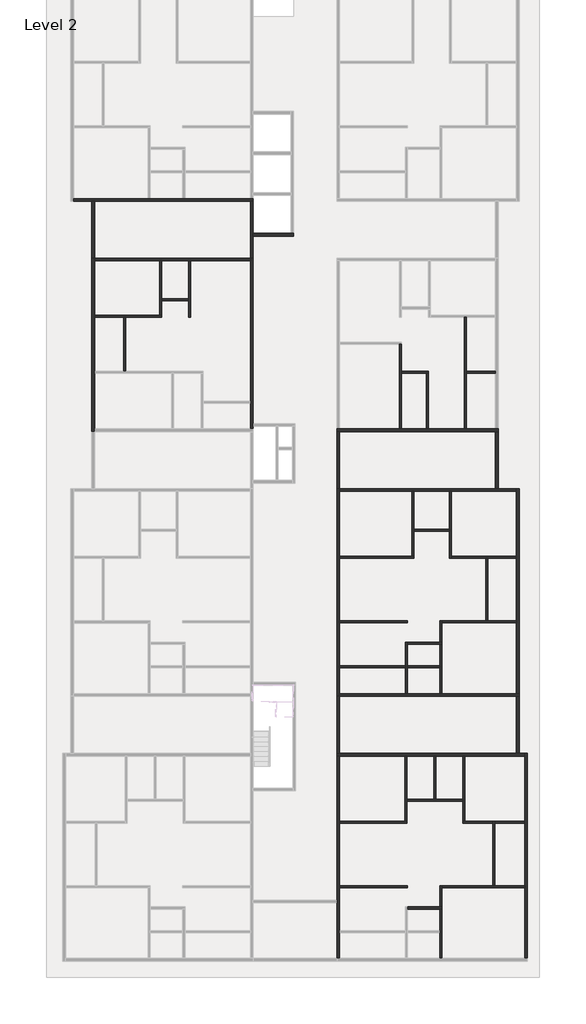
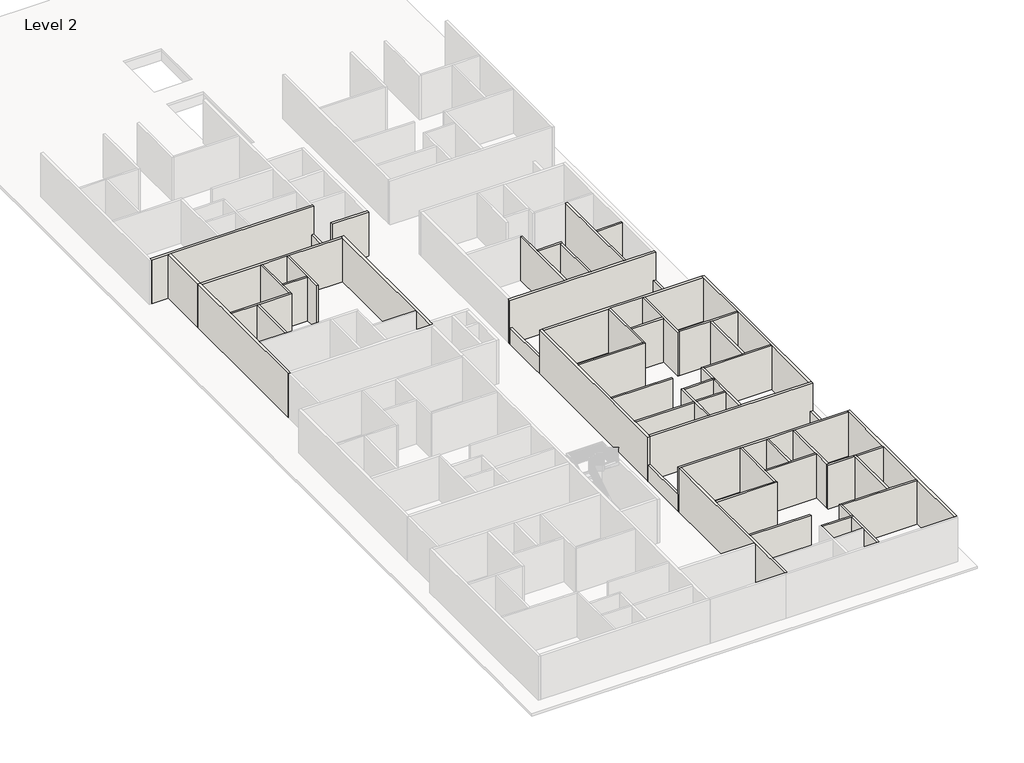
# One storey, part 2 of 8: 56 walls.
"""IFC4 building model written with IfcOpenShell, lengths in millimetres."""

from ifc_helpers import new_model, si_unit, frame, origin, place, context, project, spatial, polyline, outline, extrude, faceted_brep, element, save

model = new_model("IFC4")

# Units and contexts
model_context = context("Model", 3, world=origin())
ifc_project = project(units=[si_unit("LENGTHUNIT", "METRE", prefix="MILLI")], contexts=[model_context])

# Site, building, storey
site = spatial("IfcSite", under=ifc_project)
building = spatial("IfcBuilding", under=site)
storey = spatial("IfcBuildingStorey", under=building, Name="Level 2", Elevation=28282.6172466)

# Walls
placement = place(None, origin())
element("IfcWall", 1, ObjectType="4.5\"", at=placement, inside=storey, context=model_context, shape_type="Brep", body=[
    faceted_brep([(-12531.5544854, 2100.0216096, 28282.6172466), (-10907.2415084, 2100.0216096, 28282.6172466), (-10792.9415084, 2100.0216096, 28282.6172466), (-8759.6544854, 2100.0216096, 28282.6172466), (-8759.6544854, 2100.0216096, 31330.6172466), (-10792.9415084, 2100.0216096, 31330.6172466), (-10907.2415084, 2100.0216096, 31330.6172466), (-12531.5544854, 2100.0216096, 31330.6172466), (-12531.5544854, 2214.3216096, 28282.6172466), (-12531.5544854, 2214.3216096, 31330.6172466), (-8873.9544854, 2214.3216096, 31330.6172466), (-8759.6544854, 2214.3216096, 31330.6172466), (-8759.6544854, 2214.3216096, 28282.6172466), (-8873.9544854, 2214.3216096, 28282.6172466)], [[[0, 1, 2, 3, 4, 5, 6, 7]], [[8, 9, 10, 11, 12, 13]], [[3, 2, 1, 0, 8, 13, 12]], [[0, 7, 9, 8]], [[4, 3, 12, 11]], [[7, 6, 5, 4, 11, 10, 9]]]),
])
element("IfcWall", 2, ObjectType="4.5\"", at=placement, inside=storey, context=model_context, shape_type="Brep", body=[
    faceted_brep([(-8759.6544854, 2214.3216096, 28282.6172466), (-8759.6544854, 3014.4216096, 28282.6172466), (-8759.6544854, 3128.7216096, 28282.6172466), (-8759.6544854, 5264.2743917, 28282.6172466), (-8759.6544854, 5264.2743917, 31330.6172466), (-8759.6544854, 3128.7216096, 31330.6172466), (-8759.6544854, 3014.4216096, 31330.6172466), (-8759.6544854, 2214.3216096, 31330.6172466), (-8873.9544854, 2214.3216096, 28282.6172466), (-8873.9544854, 2214.3216096, 31330.6172466), (-8873.9544854, 5264.2743917, 31330.6172466), (-8873.9544854, 5264.2743917, 28282.6172466)], [[[0, 1, 2, 3, 4, 5, 6, 7]], [[8, 9, 10, 11]], [[3, 2, 1, 0, 8, 11]], [[0, 7, 9, 8]], [[4, 3, 11, 10]], [[7, 6, 5, 4, 10, 9]]]),
])
element("IfcWall", 3, ObjectType="4.5\"", at=placement, inside=storey, context=model_context, shape_type="Brep", body=[
    faceted_brep([(-7235.6544854, 5264.2743917, 28282.6172466), (-7235.6544854, 3128.7216096, 28282.6172466), (-7235.6544854, 3014.4216096, 28282.6172466), (-7235.6544854, 2100.0216096, 28282.6172466), (-7235.6544854, 2100.0216096, 31330.6172466), (-7235.6544854, 3014.4216096, 31330.6172466), (-7235.6544854, 3128.7216096, 31330.6172466), (-7235.6544854, 5264.2743917, 31330.6172466), (-7121.3544854, 5264.2743917, 28282.6172466), (-7121.3544854, 5264.2743917, 31330.6172466), (-7121.3544854, 2100.0216096, 31330.6172466), (-7121.3544854, 2100.0216096, 28282.6172466)], [[[0, 1, 2, 3, 4, 5, 6, 7]], [[8, 9, 10, 11]], [[3, 2, 1, 0, 8, 11]], [[4, 3, 11, 10]], [[0, 7, 9, 8]], [[7, 6, 5, 4, 10, 9]]]),
])
element("IfcWall", 4, ObjectType="4.5\"", at=placement, inside=storey, context=model_context, shape_type="SweptSolid", body=[
    extrude(outline(polyline([(-7235.6544854, 3014.4216096), (-8759.6544854, 3014.4216096), (-8759.6544854, 3128.7216096), (-7235.6544854, 3128.7216096), (-7235.6544854, 3014.4216096)])), frame((0.0, 0.0, 28282.6172466), z_axis=(0.0, 0.0, 1.0), x_axis=(1.0, 0.0, 0.0)), (0.0, 0.0, 1.0), 3048.0),
])
element("IfcWall", 5, ObjectType="4.5\"", at=placement, inside=storey, context=model_context, shape_type="SweptSolid", body=[
    extrude(outline(polyline([(-10907.2415084, -947.4344126), (-10907.2415084, 2100.0216096), (-10792.9415084, 2100.0216096), (-10792.9415084, -947.4344126), (-10907.2415084, -947.4344126)])), frame((0.0, 0.0, 28282.6172466), z_axis=(0.0, 0.0, 1.0), x_axis=(1.0, 0.0, 0.0)), (0.0, 0.0, 1.0), 3048.0),
])
element("IfcWall", 6, ObjectType="4.5\"", at=placement, inside=storey, context=model_context, shape_type="Brep", body=[
    faceted_brep([(5056.6584916, -31173.4344126, 28282.6172466), (6885.4584916, -31173.4344126, 28282.6172466), (6999.7584916, -31173.4344126, 28282.6172466), (6999.7584916, -31173.4344126, 31330.6172466), (6885.4584916, -31173.4344126, 31330.6172466), (5056.6584916, -31173.4344126, 31330.6172466), (5056.6584916, -31059.1344126, 28282.6172466), (5056.6584916, -31059.1344126, 31330.6172466), (6885.4584916, -31059.1344126, 31330.6172466), (6999.7584916, -31059.1344126, 31330.6172466), (6999.7584916, -31059.1344126, 28282.6172466), (6885.4584916, -31059.1344126, 28282.6172466)], [[[0, 1, 2, 3, 4, 5]], [[6, 7, 8, 9, 10, 11]], [[2, 1, 0, 6, 11, 10]], [[0, 5, 7, 6]], [[3, 2, 10, 9]], [[5, 4, 3, 9, 8, 7]]]),
])
element("IfcWall", 7, ObjectType="4.5\"", at=placement, inside=storey, context=model_context, shape_type="Brep", body=[
    faceted_brep([(6885.4584916, -31173.4344126, 28282.6172466), (6885.4584916, -32392.6344126, 28282.6172466), (6885.4584916, -32506.9344126, 28282.6172466), (6885.4584916, -33954.7344126, 28282.6172466), (6885.4584916, -33954.7344126, 31330.6172466), (6885.4584916, -32506.9344126, 31330.6172466), (6885.4584916, -32392.6344126, 31330.6172466), (6885.4584916, -31173.4344126, 31330.6172466), (6999.7584916, -31173.4344126, 28282.6172466), (6999.7584916, -31173.4344126, 31330.6172466), (6999.7584916, -33954.7344126, 31330.6172466), (6999.7584916, -33954.7344126, 28282.6172466)], [[[0, 1, 2, 3, 4, 5, 6, 7]], [[8, 9, 10, 11]], [[3, 2, 1, 0, 8, 11]], [[0, 7, 9, 8]], [[4, 3, 11, 10]], [[7, 6, 5, 4, 10, 9]]]),
])
element("IfcWall", 8, ObjectType="4.5\"", at=placement, inside=storey, context=model_context, shape_type="Brep", body=[
    faceted_brep([(6999.7584916, -31059.1344126, 28282.6172466), (6999.7584916, -29966.9344126, 28282.6172466), (6999.7584916, -29852.6344126, 28282.6172466), (6999.7584916, -29852.6344126, 31330.6172466), (6999.7584916, -29966.9344126, 31330.6172466), (6999.7584916, -31059.1344126, 31330.6172466), (6885.4584916, -31059.1344126, 28282.6172466), (6885.4584916, -31059.1344126, 31330.6172466), (6885.4584916, -29852.6344126, 31330.6172466), (6885.4584916, -29852.6344126, 28282.6172466)], [[[0, 1, 2, 3, 4, 5]], [[6, 7, 8, 9]], [[2, 1, 0, 6, 9]], [[0, 5, 7, 6]], [[3, 2, 9, 8]], [[5, 4, 3, 8, 7]]]),
])
element("IfcWall", 9, ObjectType="4.5\"", at=placement, inside=storey, context=model_context, shape_type="Brep", body=[
    faceted_brep([(6999.7584916, -29966.9344126, 28282.6172466), (11660.6584916, -29966.9344126, 28282.6172466), (11660.6584916, -29966.9344126, 31330.6172466), (6999.7584916, -29966.9344126, 31330.6172466), (6999.7584916, -29852.6344126, 28282.6172466), (6999.7584916, -29852.6344126, 31330.6172466), (9869.9584916, -29852.6344126, 31330.6172466), (9984.2584916, -29852.6344126, 31330.6172466), (11660.6584916, -29852.6344126, 31330.6172466), (11660.6584916, -29852.6344126, 28282.6172466), (9984.2584916, -29852.6344126, 28282.6172466), (9869.9584916, -29852.6344126, 28282.6172466)], [[[0, 1, 2, 3]], [[4, 5, 6, 7, 8, 9, 10, 11]], [[1, 0, 4, 11, 10, 9]], [[0, 3, 5, 4]], [[2, 1, 9, 8]], [[3, 2, 8, 7, 6, 5]]]),
])
element("IfcWall", 10, ObjectType="4.5\"", at=placement, inside=storey, context=model_context, shape_type="SweptSolid", body=[
    extrude(outline(polyline([(5056.6584916, -29966.9344126), (1259.3584916, -29966.9344126), (1259.3584916, -29852.6344126), (5056.6584916, -29852.6344126), (5056.6584916, -29966.9344126)])), frame((0.0, 0.0, 28282.6172466), z_axis=(0.0, 0.0, 1.0), x_axis=(1.0, 0.0, 0.0)), (0.0, 0.0, 1.0), 3048.0),
])
element("IfcWall", 11, ObjectType="4.5\"", at=placement, inside=storey, context=model_context, shape_type="Brep", body=[
    faceted_brep([(1259.3584916, -26347.4344126, 28282.6172466), (5031.2584916, -26347.4344126, 28282.6172466), (5031.2584916, -26347.4344126, 31330.6172466), (1259.3584916, -26347.4344126, 31330.6172466), (1259.3584916, -26233.1344126, 28282.6172466), (1259.3584916, -26233.1344126, 31330.6172466), (4916.9584916, -26233.1344126, 31330.6172466), (5031.2584916, -26233.1344126, 31330.6172466), (5031.2584916, -26233.1344126, 28282.6172466), (4916.9584916, -26233.1344126, 28282.6172466)], [[[0, 1, 2, 3]], [[4, 5, 6, 7, 8, 9]], [[1, 0, 4, 9, 8]], [[0, 3, 5, 4]], [[2, 1, 8, 7]], [[3, 2, 7, 6, 5]]]),
])
element("IfcWall", 12, ObjectType="4.5\"", at=placement, inside=storey, context=model_context, shape_type="Brep", body=[
    faceted_brep([(5031.2584916, -26233.1344126, 28282.6172466), (5031.2584916, -25128.2344126, 28282.6172466), (5031.2584916, -25013.9344126, 28282.6172466), (5031.2584916, -22575.5344126, 28282.6172466), (5031.2584916, -22575.5344126, 31330.6172466), (5031.2584916, -25013.9344126, 31330.6172466), (5031.2584916, -25128.2344126, 31330.6172466), (5031.2584916, -26233.1344126, 31330.6172466), (4916.9584916, -26233.1344126, 28282.6172466), (4916.9584916, -26233.1344126, 31330.6172466), (4916.9584916, -22575.5344126, 31330.6172466), (4916.9584916, -22575.5344126, 28282.6172466)], [[[0, 1, 2, 3, 4, 5, 6, 7]], [[8, 9, 10, 11]], [[3, 2, 1, 0, 8, 11]], [[0, 7, 9, 8]], [[4, 3, 11, 10]], [[7, 6, 5, 4, 10, 9]]]),
])
element("IfcWall", 13, ObjectType="4.5\"", at=placement, inside=storey, context=model_context, shape_type="Brep", body=[
    faceted_brep([(9984.2584916, -29852.6344126, 28282.6172466), (9984.2584916, -26347.4344126, 28282.6172466), (9984.2584916, -26233.1344126, 28282.6172466), (9984.2584916, -26233.1344126, 31330.6172466), (9984.2584916, -26347.4344126, 31330.6172466), (9984.2584916, -29852.6344126, 31330.6172466), (9869.9584916, -29852.6344126, 28282.6172466), (9869.9584916, -29852.6344126, 31330.6172466), (9869.9584916, -26347.4344126, 31330.6172466), (9869.9584916, -26233.1344126, 31330.6172466), (9869.9584916, -26233.1344126, 28282.6172466), (9869.9584916, -26347.4344126, 28282.6172466)], [[[0, 1, 2, 3, 4, 5]], [[6, 7, 8, 9, 10, 11]], [[2, 1, 0, 6, 11, 10]], [[0, 5, 7, 6]], [[3, 2, 10, 9]], [[5, 4, 3, 9, 8, 7]]]),
])
element("IfcWall", 14, ObjectType="4.5\"", at=placement, inside=storey, context=model_context, shape_type="SweptSolid", body=[
    extrude(outline(polyline([(11660.6584916, -26347.4344126), (9984.2584916, -26347.4344126), (9984.2584916, -26233.1344126), (11660.6584916, -26233.1344126), (11660.6584916, -26347.4344126)])), frame((0.0, 0.0, 28282.6172466), z_axis=(0.0, 0.0, 1.0), x_axis=(1.0, 0.0, 0.0)), (0.0, 0.0, 1.0), 3048.0),
])
element("IfcWall", 15, ObjectType="4.5\"", at=placement, inside=storey, context=model_context, shape_type="Brep", body=[
    faceted_brep([(9869.9584916, -26233.1344126, 28282.6172466), (8307.8584916, -26233.1344126, 28282.6172466), (8193.5584916, -26233.1344126, 28282.6172466), (8193.5584916, -26233.1344126, 31330.6172466), (8307.8584916, -26233.1344126, 31330.6172466), (9869.9584916, -26233.1344126, 31330.6172466), (9869.9584916, -26347.4344126, 28282.6172466), (9869.9584916, -26347.4344126, 31330.6172466), (8193.5584916, -26347.4344126, 31330.6172466), (8193.5584916, -26347.4344126, 28282.6172466)], [[[0, 1, 2, 3, 4, 5]], [[6, 7, 8, 9]], [[2, 1, 0, 6, 9]], [[0, 5, 7, 6]], [[3, 2, 9, 8]], [[5, 4, 3, 8, 7]]]),
])
element("IfcWall", 16, ObjectType="4.5\"", at=placement, inside=storey, context=model_context, shape_type="Brep", body=[
    faceted_brep([(8307.8584916, -26233.1344126, 28282.6172466), (8307.8584916, -22575.5344126, 28282.6172466), (8307.8584916, -22575.5344126, 31330.6172466), (8307.8584916, -26233.1344126, 31330.6172466), (8193.5584916, -26233.1344126, 28282.6172466), (8193.5584916, -26233.1344126, 31330.6172466), (8193.5584916, -25128.2344126, 31330.6172466), (8193.5584916, -25013.9344126, 31330.6172466), (8193.5584916, -22575.5344126, 31330.6172466), (8193.5584916, -22575.5344126, 28282.6172466), (8193.5584916, -25013.9344126, 28282.6172466), (8193.5584916, -25128.2344126, 28282.6172466)], [[[0, 1, 2, 3]], [[4, 5, 6, 7, 8, 9, 10, 11]], [[1, 0, 4, 11, 10, 9]], [[0, 3, 5, 4]], [[2, 1, 9, 8]], [[3, 2, 8, 7, 6, 5]]]),
])
element("IfcWall", 17, ObjectType="4.5\"", at=placement, inside=storey, context=model_context, shape_type="Brep", body=[
    faceted_brep([(5031.2584916, -25128.2344126, 28282.6172466), (8193.5584916, -25128.2344126, 28282.6172466), (8193.5584916, -25128.2344126, 31330.6172466), (5031.2584916, -25128.2344126, 31330.6172466), (5031.2584916, -25013.9344126, 28282.6172466), (5031.2584916, -25013.9344126, 31330.6172466), (6555.2584916, -25013.9344126, 31330.6172466), (6669.5584916, -25013.9344126, 31330.6172466), (8193.5584916, -25013.9344126, 31330.6172466), (8193.5584916, -25013.9344126, 28282.6172466), (6669.5584916, -25013.9344126, 28282.6172466), (6555.2584916, -25013.9344126, 28282.6172466)], [[[0, 1, 2, 3]], [[4, 5, 6, 7, 8, 9, 10, 11]], [[1, 0, 4, 11, 10, 9]], [[0, 3, 5, 4]], [[2, 1, 9, 8]], [[3, 2, 8, 7, 6, 5]]]),
])
element("IfcWall", 18, ObjectType="4.5\"", at=placement, inside=storey, context=model_context, shape_type="SweptSolid", body=[
    extrude(outline(polyline([(6555.2584916, -25013.9344126), (6555.2584916, -22575.5344126), (6669.5584916, -22575.5344126), (6669.5584916, -25013.9344126), (6555.2584916, -25013.9344126)])), frame((0.0, 0.0, 28282.6172466), z_axis=(0.0, 0.0, 1.0), x_axis=(1.0, 0.0, 0.0)), (0.0, 0.0, 1.0), 3048.0),
])
element("IfcWall", 19, ObjectType="4.5\"", at=placement, inside=storey, context=model_context, shape_type="SweptSolid", body=[
    extrude(outline(polyline([(4942.3584916, -17622.5344126), (1259.3584916, -17622.5344126), (1259.3584916, -17508.2344126), (4942.3584916, -17508.2344126), (4942.3584916, -17622.5344126)])), frame((0.0, 0.0, 28282.6172466), z_axis=(0.0, 0.0, 1.0), x_axis=(1.0, 0.0, 0.0)), (0.0, 0.0, 1.0), 3048.0),
])
element("IfcWall", 20, ObjectType="4.5\"", at=placement, inside=storey, context=model_context, shape_type="Brep", body=[
    faceted_brep([(4942.3584916, -16174.7344126, 28282.6172466), (4942.3584916, -17508.2344126, 28282.6172466), (4942.3584916, -17622.5344126, 28282.6172466), (4942.3584916, -19070.3344126, 28282.6172466), (4942.3584916, -19070.3344126, 31330.6172466), (4942.3584916, -17622.5344126, 31330.6172466), (4942.3584916, -17508.2344126, 31330.6172466), (4942.3584916, -16174.7344126, 31330.6172466), (5056.6584916, -16174.7344126, 28282.6172466), (5056.6584916, -16174.7344126, 31330.6172466), (5056.6584916, -16289.0344126, 31330.6172466), (5056.6584916, -17508.2344126, 31330.6172466), (5056.6584916, -17622.5344126, 31330.6172466), (5056.6584916, -19070.3344126, 31330.6172466), (5056.6584916, -19070.3344126, 28282.6172466), (5056.6584916, -17622.5344126, 28282.6172466), (5056.6584916, -17508.2344126, 28282.6172466), (5056.6584916, -16289.0344126, 28282.6172466)], [[[0, 1, 2, 3, 4, 5, 6, 7]], [[8, 9, 10, 11, 12, 13, 14, 15, 16, 17]], [[3, 2, 1, 0, 8, 17, 16, 15, 14]], [[4, 3, 14, 13]], [[0, 7, 9, 8]], [[7, 6, 5, 4, 13, 12, 11, 10, 9]]]),
])
element("IfcWall", 21, ObjectType="4.5\"", at=placement, inside=storey, context=model_context, shape_type="Brep", body=[
    faceted_brep([(5056.6584916, -16289.0344126, 28282.6172466), (6885.4584916, -16289.0344126, 28282.6172466), (6999.7584916, -16289.0344126, 28282.6172466), (6999.7584916, -16289.0344126, 31330.6172466), (6885.4584916, -16289.0344126, 31330.6172466), (5056.6584916, -16289.0344126, 31330.6172466), (5056.6584916, -16174.7344126, 28282.6172466), (5056.6584916, -16174.7344126, 31330.6172466), (6885.4584916, -16174.7344126, 31330.6172466), (6999.7584916, -16174.7344126, 31330.6172466), (6999.7584916, -16174.7344126, 28282.6172466), (6885.4584916, -16174.7344126, 28282.6172466)], [[[0, 1, 2, 3, 4, 5]], [[6, 7, 8, 9, 10, 11]], [[2, 1, 0, 6, 11, 10]], [[0, 5, 7, 6]], [[3, 2, 10, 9]], [[5, 4, 3, 9, 8, 7]]]),
])
element("IfcWall", 22, ObjectType="4.5\"", at=placement, inside=storey, context=model_context, shape_type="Brep", body=[
    faceted_brep([(6885.4584916, -16289.0344126, 28282.6172466), (6885.4584916, -17508.2344126, 28282.6172466), (6885.4584916, -17622.5344126, 28282.6172466), (6885.4584916, -19070.3344126, 28282.6172466), (6885.4584916, -19070.3344126, 31330.6172466), (6885.4584916, -17622.5344126, 31330.6172466), (6885.4584916, -17508.2344126, 31330.6172466), (6885.4584916, -16289.0344126, 31330.6172466), (6999.7584916, -16289.0344126, 28282.6172466), (6999.7584916, -16289.0344126, 31330.6172466), (6999.7584916, -19070.3344126, 31330.6172466), (6999.7584916, -19070.3344126, 28282.6172466)], [[[0, 1, 2, 3, 4, 5, 6, 7]], [[8, 9, 10, 11]], [[3, 2, 1, 0, 8, 11]], [[0, 7, 9, 8]], [[4, 3, 11, 10]], [[7, 6, 5, 4, 10, 9]]]),
])
element("IfcWall", 23, ObjectType="4.5\"", at=placement, inside=storey, context=model_context, shape_type="SweptSolid", body=[
    extrude(outline(polyline([(6885.4584916, -17622.5344126), (5056.6584916, -17622.5344126), (5056.6584916, -17508.2344126), (6885.4584916, -17508.2344126), (6885.4584916, -17622.5344126)])), frame((0.0, 0.0, 28282.6172466), z_axis=(0.0, 0.0, 1.0), x_axis=(1.0, 0.0, 0.0)), (0.0, 0.0, 1.0), 3048.0),
])
element("IfcWall", 24, ObjectType="4.5\"", at=placement, inside=storey, context=model_context, shape_type="Brep", body=[
    faceted_brep([(6999.7584916, -16174.7344126, 28282.6172466), (6999.7584916, -15082.5344126, 28282.6172466), (6999.7584916, -14968.2344126, 28282.6172466), (6999.7584916, -14968.2344126, 31330.6172466), (6999.7584916, -15082.5344126, 31330.6172466), (6999.7584916, -16174.7344126, 31330.6172466), (6885.4584916, -16174.7344126, 28282.6172466), (6885.4584916, -16174.7344126, 31330.6172466), (6885.4584916, -14968.2344126, 31330.6172466), (6885.4584916, -14968.2344126, 28282.6172466)], [[[0, 1, 2, 3, 4, 5]], [[6, 7, 8, 9]], [[2, 1, 0, 6, 9]], [[0, 5, 7, 6]], [[3, 2, 9, 8]], [[5, 4, 3, 8, 7]]]),
])
element("IfcWall", 25, ObjectType="4.5\"", at=placement, inside=storey, context=model_context, shape_type="Brep", body=[
    faceted_brep([(6999.7584916, -15082.5344126, 28282.6172466), (11208.5214687, -15082.5344126, 28282.6172466), (11208.5214687, -15082.5344126, 31330.6172466), (6999.7584916, -15082.5344126, 31330.6172466), (6999.7584916, -14968.2344126, 28282.6172466), (6999.7584916, -14968.2344126, 31330.6172466), (9469.9084916, -14968.2344126, 31330.6172466), (9584.2084916, -14968.2344126, 31330.6172466), (11208.5214687, -14968.2344126, 31330.6172466), (11208.5214687, -14968.2344126, 28282.6172466), (9584.2084916, -14968.2344126, 28282.6172466), (9469.9084916, -14968.2344126, 28282.6172466)], [[[0, 1, 2, 3]], [[4, 5, 6, 7, 8, 9, 10, 11]], [[1, 0, 4, 11, 10, 9]], [[0, 3, 5, 4]], [[2, 1, 9, 8]], [[3, 2, 8, 7, 6, 5]]]),
])
element("IfcWall", 26, ObjectType="4.5\"", at=placement, inside=storey, context=model_context, shape_type="SweptSolid", body=[
    extrude(outline(polyline([(5056.6584916, -15082.5344126), (1259.3584916, -15082.5344126), (1259.3584916, -14968.2344126), (5056.6584916, -14968.2344126), (5056.6584916, -15082.5344126)])), frame((0.0, 0.0, 28282.6172466), z_axis=(0.0, 0.0, 1.0), x_axis=(1.0, 0.0, 0.0)), (0.0, 0.0, 1.0), 3048.0),
])
element("IfcWall", 27, ObjectType="4.5\"", at=placement, inside=storey, context=model_context, shape_type="Brep", body=[
    faceted_brep([(1259.3584916, -11463.0344126, 28282.6172466), (5430.0214687, -11463.0344126, 28282.6172466), (5430.0214687, -11463.0344126, 31330.6172466), (1259.3584916, -11463.0344126, 31330.6172466), (1259.3584916, -11348.7344126, 28282.6172466), (1259.3584916, -11348.7344126, 31330.6172466), (5315.7214687, -11348.7344126, 31330.6172466), (5430.0214687, -11348.7344126, 31330.6172466), (5430.0214687, -11348.7344126, 28282.6172466), (5315.7214687, -11348.7344126, 28282.6172466)], [[[0, 1, 2, 3]], [[4, 5, 6, 7, 8, 9]], [[1, 0, 4, 9, 8]], [[0, 3, 5, 4]], [[2, 1, 8, 7]], [[3, 2, 7, 6, 5]]]),
])
element("IfcWall", 28, ObjectType="4.5\"", at=placement, inside=storey, context=model_context, shape_type="Brep", body=[
    faceted_brep([(5430.0214687, -11348.7344126, 28282.6172466), (5430.0214687, -9939.0344126, 28282.6172466), (5430.0214687, -9824.7344126, 28282.6172466), (5430.0214687, -7691.1344126, 28282.6172466), (5430.0214687, -7691.1344126, 31330.6172466), (5430.0214687, -9824.7344126, 31330.6172466), (5430.0214687, -9939.0344126, 31330.6172466), (5430.0214687, -11348.7344126, 31330.6172466), (5315.7214687, -11348.7344126, 28282.6172466), (5315.7214687, -11348.7344126, 31330.6172466), (5315.7214687, -7691.1344126, 31330.6172466), (5315.7214687, -7691.1344126, 28282.6172466)], [[[0, 1, 2, 3, 4, 5, 6, 7]], [[8, 9, 10, 11]], [[3, 2, 1, 0, 8, 11]], [[0, 7, 9, 8]], [[4, 3, 11, 10]], [[7, 6, 5, 4, 10, 9]]]),
])
element("IfcWall", 29, ObjectType="4.5\"", at=placement, inside=storey, context=model_context, shape_type="SweptSolid", body=[
    extrude(outline(polyline([(7436.6214687, -9939.0344126), (5430.0214687, -9939.0344126), (5430.0214687, -9824.7344126), (7436.6214687, -9824.7344126), (7436.6214687, -9939.0344126)])), frame((0.0, 0.0, 28282.6172466), z_axis=(0.0, 0.0, 1.0), x_axis=(1.0, 0.0, 0.0)), (0.0, 0.0, 1.0), 3048.0),
])
element("IfcWall", 30, ObjectType="4.5\"", at=placement, inside=storey, context=model_context, shape_type="Brep", body=[
    faceted_brep([(7436.6214687, -7691.1344126, 28282.6172466), (7436.6214687, -9824.7344126, 28282.6172466), (7436.6214687, -9939.0344126, 28282.6172466), (7436.6214687, -11463.0344126, 28282.6172466), (7436.6214687, -11463.0344126, 31330.6172466), (7436.6214687, -9939.0344126, 31330.6172466), (7436.6214687, -9824.7344126, 31330.6172466), (7436.6214687, -7691.1344126, 31330.6172466), (7550.9214687, -7691.1344126, 28282.6172466), (7550.9214687, -7691.1344126, 31330.6172466), (7550.9214687, -11348.7344126, 31330.6172466), (7550.9214687, -11463.0344126, 31330.6172466), (7550.9214687, -11463.0344126, 28282.6172466), (7550.9214687, -11348.7344126, 28282.6172466)], [[[0, 1, 2, 3, 4, 5, 6, 7]], [[8, 9, 10, 11, 12, 13]], [[3, 2, 1, 0, 8, 13, 12]], [[0, 7, 9, 8]], [[4, 3, 12, 11]], [[7, 6, 5, 4, 11, 10, 9]]]),
])
element("IfcWall", 31, ObjectType="4.5\"", at=placement, inside=storey, context=model_context, shape_type="Brep", body=[
    faceted_brep([(7550.9214687, -11463.0344126, 28282.6172466), (9469.9084916, -11463.0344126, 28282.6172466), (9584.2084916, -11463.0344126, 28282.6172466), (11208.5214687, -11463.0344126, 28282.6172466), (11208.5214687, -11463.0344126, 31330.6172466), (9584.2084916, -11463.0344126, 31330.6172466), (9469.9084916, -11463.0344126, 31330.6172466), (7550.9214687, -11463.0344126, 31330.6172466), (7550.9214687, -11348.7344126, 28282.6172466), (7550.9214687, -11348.7344126, 31330.6172466), (11208.5214687, -11348.7344126, 31330.6172466), (11208.5214687, -11348.7344126, 28282.6172466)], [[[0, 1, 2, 3, 4, 5, 6, 7]], [[8, 9, 10, 11]], [[3, 2, 1, 0, 8, 11]], [[0, 7, 9, 8]], [[4, 3, 11, 10]], [[7, 6, 5, 4, 10, 9]]]),
])
element("IfcWall", 32, ObjectType="4.5\"", at=placement, inside=storey, context=model_context, shape_type="SweptSolid", body=[
    extrude(outline(polyline([(9469.9084916, -14968.2344126), (9469.9084916, -11463.0344126), (9584.2084916, -11463.0344126), (9584.2084916, -14968.2344126), (9469.9084916, -14968.2344126)])), frame((0.0, 0.0, 28282.6172466), z_axis=(0.0, 0.0, 1.0), x_axis=(1.0, 0.0, 0.0)), (0.0, 0.0, 1.0), 3048.0),
])
element("IfcWall", 33, ObjectType="4.5\"", at=placement, inside=storey, context=model_context, shape_type="Brep", body=[
    faceted_brep([(4610.8714687, 572.7745083, 28282.6172466), (4610.8714687, -4185.9344126, 28282.6172466), (4610.8714687, -4185.9344126, 31330.6172466), (4610.8714687, 572.7745083, 31330.6172466), (4725.1714687, 572.7745083, 28282.6172466), (4725.1714687, 572.7745083, 31330.6172466), (4725.1714687, -947.4344126, 31330.6172466), (4725.1714687, -1061.7344126, 31330.6172466), (4725.1714687, -4185.9344126, 31330.6172466), (4725.1714687, -4185.9344126, 28282.6172466), (4725.1714687, -1061.7344126, 28282.6172466), (4725.1714687, -947.4344126, 28282.6172466)], [[[0, 1, 2, 3]], [[4, 5, 6, 7, 8, 9, 10, 11]], [[1, 0, 4, 11, 10, 9]], [[0, 3, 5, 4]], [[2, 1, 9, 8]], [[3, 2, 8, 7, 6, 5]]]),
])
element("IfcWall", 34, ObjectType="4.5\"", at=placement, inside=storey, context=model_context, shape_type="Brep", body=[
    faceted_brep([(4725.1714687, -1061.7344126, 28282.6172466), (6134.8714687, -1061.7344126, 28282.6172466), (6249.1714687, -1061.7344126, 28282.6172466), (6249.1714687, -1061.7344126, 31330.6172466), (6134.8714687, -1061.7344126, 31330.6172466), (4725.1714687, -1061.7344126, 31330.6172466), (4725.1714687, -947.4344126, 28282.6172466), (4725.1714687, -947.4344126, 31330.6172466), (6249.1714687, -947.4344126, 31330.6172466), (6249.1714687, -947.4344126, 28282.6172466)], [[[0, 1, 2, 3, 4, 5]], [[6, 7, 8, 9]], [[2, 1, 0, 6, 9]], [[0, 5, 7, 6]], [[3, 2, 9, 8]], [[5, 4, 3, 8, 7]]]),
])
element("IfcWall", 35, ObjectType="4.5\"", at=placement, inside=storey, context=model_context, shape_type="SweptSolid", body=[
    extrude(outline(polyline([(6134.8714687, -4185.9344126), (6134.8714687, -1061.7344126), (6249.1714687, -1061.7344126), (6249.1714687, -4185.9344126), (6134.8714687, -4185.9344126)])), frame((0.0, 0.0, 28282.6172466), z_axis=(0.0, 0.0, 1.0), x_axis=(1.0, 0.0, 0.0)), (0.0, 0.0, 1.0), 3048.0),
])
element("IfcWall", 36, ObjectType="4.5\"", at=placement, inside=storey, context=model_context, shape_type="Brep", body=[
    faceted_brep([(8396.7584916, -4185.9344126, 28282.6172466), (8396.7584916, -1061.7344126, 28282.6172466), (8396.7584916, -947.4344126, 28282.6172466), (8396.7584916, 2100.0216096, 28282.6172466), (8396.7584916, 2100.0216096, 31330.6172466), (8396.7584916, -947.4344126, 31330.6172466), (8396.7584916, -1061.7344126, 31330.6172466), (8396.7584916, -4185.9344126, 31330.6172466), (8282.4584916, -4185.9344126, 28282.6172466), (8282.4584916, -4185.9344126, 31330.6172466), (8282.4584916, 2100.0216096, 31330.6172466), (8282.4584916, 2100.0216096, 28282.6172466)], [[[0, 1, 2, 3, 4, 5, 6, 7]], [[8, 9, 10, 11]], [[3, 2, 1, 0, 8, 11]], [[0, 7, 9, 8]], [[4, 3, 11, 10]], [[7, 6, 5, 4, 10, 9]]]),
])
element("IfcWall", 37, ObjectType="4.5\"", at=placement, inside=storey, context=model_context, shape_type="SweptSolid", body=[
    extrude(outline(polyline([(8396.7584916, -947.4344126), (10021.0714687, -947.4344126), (10021.0714687, -1061.7344126), (8396.7584916, -1061.7344126), (8396.7584916, -947.4344126)])), frame((0.0, 0.0, 28282.6172466), z_axis=(0.0, 0.0, 1.0), x_axis=(1.0, 0.0, 0.0)), (0.0, 0.0, 1.0), 3048.0),
])
element("IfcWall", 38, ObjectType="6\"", at=placement, inside=storey, context=model_context, shape_type="Brep", body=[
    faceted_brep([(-13719.0044854, 8615.1216096, 28282.6172466), (-12683.9544854, 8615.1216096, 28282.6172466), (-12531.5544854, 8615.1216096, 28282.6172466), (-3769.8415084, 8615.1216096, 28282.6172466), (-3617.4415084, 8615.1216096, 28282.6172466), (-3617.4415084, 8615.1216096, 29501.8172466), (-3617.4415084, 8615.1216096, 31330.6172466), (-12531.5544854, 8615.1216096, 31330.6172466), (-12683.9544854, 8615.1216096, 31330.6172466), (-13719.0044854, 8615.1216096, 31330.6172466), (-13719.0044854, 8767.5216096, 28282.6172466), (-13719.0044854, 8767.5216096, 31330.6172466), (-9510.2415084, 8767.5216096, 31330.6172466), (-9395.9415084, 8767.5216096, 31330.6172466), (-7567.1415084, 8767.5216096, 31330.6172466), (-7452.8415084, 8767.5216096, 31330.6172466), (-3769.8415084, 8767.5216096, 31330.6172466), (-3617.4415084, 8767.5216096, 31330.6172466), (-3617.4415084, 8767.5216096, 28282.6172466), (-3769.8415084, 8767.5216096, 28282.6172466), (-7452.8415084, 8767.5216096, 28282.6172466), (-7567.1415084, 8767.5216096, 28282.6172466), (-9395.9415084, 8767.5216096, 28282.6172466), (-9510.2415084, 8767.5216096, 28282.6172466)], [[[0, 1, 2, 3, 4, 5, 6, 7, 8, 9]], [[10, 11, 12, 13, 14, 15, 16, 17, 18, 19, 20, 21, 22, 23]], [[4, 3, 2, 1, 0, 10, 23, 22, 21, 20, 19, 18]], [[0, 9, 11, 10]], [[4, 18, 17, 6, 5]], [[9, 8, 7, 6, 17, 16, 15, 14, 13, 12, 11]]]),
])
element("IfcWall", 39, ObjectType="6\"", at=placement, inside=storey, context=model_context, shape_type="Brep", body=[
    faceted_brep([(-12683.9544854, 5416.6743917, 28282.6172466), (-12683.9544854, -4338.3344126, 28282.6172466), (-12683.9544854, -4338.3344126, 31330.6172466), (-12683.9544854, 5416.6743917, 31330.6172466), (-12531.5544854, 5416.6743917, 28282.6172466), (-12531.5544854, 5416.6743917, 31330.6172466), (-12531.5544854, 5264.2743917, 31330.6172466), (-12531.5544854, 2214.3216096, 31330.6172466), (-12531.5544854, 2100.0216096, 31330.6172466), (-12531.5544854, -947.4344126, 31330.6172466), (-12531.5544854, -1061.7344126, 31330.6172466), (-12531.5544854, -4185.9344126, 31330.6172466), (-12531.5544854, -4338.3344126, 31330.6172466), (-12531.5544854, -4338.3344126, 28282.6172466), (-12531.5544854, -4185.9344126, 28282.6172466), (-12531.5544854, -1061.7344126, 28282.6172466), (-12531.5544854, -947.4344126, 28282.6172466), (-12531.5544854, 2100.0216096, 28282.6172466), (-12531.5544854, 2214.3216096, 28282.6172466), (-12531.5544854, 5264.2743917, 28282.6172466)], [[[0, 1, 2, 3]], [[4, 5, 6, 7, 8, 9, 10, 11, 12, 13, 14, 15, 16, 17, 18, 19]], [[1, 0, 4, 19, 18, 17, 16, 15, 14, 13]], [[2, 1, 13, 12]], [[0, 3, 5, 4]], [[3, 2, 12, 11, 10, 9, 8, 7, 6, 5]]]),
])
element("IfcWall", 40, ObjectType="6\"", at=placement, inside=storey, context=model_context, shape_type="Brep", body=[
    faceted_brep([(-3617.4415084, -4185.9344126, 28282.6172466), (-3617.4415084, -4034.6751812, 28282.6172466), (-3617.4415084, -3882.2751812, 28282.6172466), (-3617.4415084, 5416.6743917, 28282.6172466), (-3617.4415084, 5416.6743917, 31330.6172466), (-3617.4415084, -3882.2751812, 31330.6172466), (-3617.4415084, -4034.6751812, 31330.6172466), (-3617.4415084, -4185.9344126, 31330.6172466), (-3769.8415084, -4185.9344126, 28282.6172466), (-3769.8415084, -4185.9344126, 31330.6172466), (-3769.8415084, -2738.1344126, 31330.6172466), (-3769.8415084, -2623.8344126, 31330.6172466), (-3769.8415084, 5264.2743917, 31330.6172466), (-3769.8415084, 5416.6743917, 31330.6172466), (-3769.8415084, 5416.6743917, 28282.6172466), (-3769.8415084, 5264.2743917, 28282.6172466), (-3769.8415084, -2623.8344126, 28282.6172466), (-3769.8415084, -2738.1344126, 28282.6172466)], [[[0, 1, 2, 3, 4, 5, 6, 7]], [[8, 9, 10, 11, 12, 13, 14, 15, 16, 17]], [[3, 2, 1, 0, 8, 17, 16, 15, 14]], [[0, 7, 9, 8]], [[3, 14, 13, 4]], [[7, 6, 5, 4, 13, 12, 11, 10, 9]]]),
])
element("IfcWall", 41, ObjectType="6\"", at=placement, inside=storey, context=model_context, shape_type="Brep", body=[
    faceted_brep([(-3769.8415084, 5416.6743917, 31330.6172466), (-3769.8415084, 5416.6743917, 28282.6172466), (-12531.5544854, 5416.6743917, 28282.6172466), (-12531.5544854, 5416.6743917, 31330.6172466), (-3769.8415084, 5264.2743917, 28282.6172466), (-3769.8415084, 5264.2743917, 31330.6172466), (-7121.3544854, 5264.2743917, 31330.6172466), (-7235.6544854, 5264.2743917, 31330.6172466), (-8759.6544854, 5264.2743917, 31330.6172466), (-8873.9544854, 5264.2743917, 31330.6172466), (-12531.5544854, 5264.2743917, 31330.6172466), (-12531.5544854, 5264.2743917, 28282.6172466), (-8873.9544854, 5264.2743917, 28282.6172466), (-8759.6544854, 5264.2743917, 28282.6172466), (-7235.6544854, 5264.2743917, 28282.6172466), (-7121.3544854, 5264.2743917, 28282.6172466)], [[[0, 1, 2, 3]], [[4, 5, 6, 7, 8, 9, 10, 11, 12, 13, 14, 15]], [[2, 1, 4, 15, 14, 13, 12, 11]], [[3, 2, 11, 10]], [[0, 5, 4, 1]], [[0, 3, 10, 9, 8, 7, 6, 5]]]),
])
element("IfcWall", 42, ObjectType="6\"", at=placement, inside=storey, context=model_context, shape_type="Brep", body=[
    faceted_brep([(11813.0584916, -33954.7344126, 28282.6172466), (11813.0584916, -22423.1344126, 28282.6172466), (11813.0584916, -22423.1344126, 31330.6172466), (11813.0584916, -33954.7344126, 31330.6172466), (11660.6584916, -33954.7344126, 28282.6172466), (11660.6584916, -33954.7344126, 31330.6172466), (11660.6584916, -29966.9344126, 31330.6172466), (11660.6584916, -29852.6344126, 31330.6172466), (11660.6584916, -26347.4344126, 31330.6172466), (11660.6584916, -26233.1344126, 31330.6172466), (11660.6584916, -22575.5344126, 31330.6172466), (11660.6584916, -22423.1344126, 31330.6172466), (11660.6584916, -22423.1344126, 28282.6172466), (11660.6584916, -22575.5344126, 28282.6172466), (11660.6584916, -26233.1344126, 28282.6172466), (11660.6584916, -26347.4344126, 28282.6172466), (11660.6584916, -29852.6344126, 28282.6172466), (11660.6584916, -29966.9344126, 28282.6172466)], [[[0, 1, 2, 3]], [[4, 5, 6, 7, 8, 9, 10, 11, 12, 13, 14, 15, 16, 17]], [[1, 0, 4, 17, 16, 15, 14, 13, 12]], [[0, 3, 5, 4]], [[2, 1, 12, 11]], [[3, 2, 11, 10, 9, 8, 7, 6, 5]]]),
])
element("IfcWall", 43, ObjectType="6\"", at=placement, inside=storey, context=model_context, shape_type="Brep", body=[
    faceted_brep([(11660.6584916, -22423.1344126, 28282.6172466), (11360.9214687, -22423.1344126, 28282.6172466), (11208.5214687, -22423.1344126, 28282.6172466), (1259.3584916, -22423.1344126, 28282.6172466), (1106.9584916, -22423.1344126, 28282.6172466), (1106.9584916, -22423.1344126, 29501.8172466), (1106.9584916, -22423.1344126, 31330.6172466), (11660.6584916, -22423.1344126, 31330.6172466), (11660.6584916, -22575.5344126, 28282.6172466), (11660.6584916, -22575.5344126, 31330.6172466), (8307.8584916, -22575.5344126, 31330.6172466), (8193.5584916, -22575.5344126, 31330.6172466), (6669.5584916, -22575.5344126, 31330.6172466), (6555.2584916, -22575.5344126, 31330.6172466), (5031.2584916, -22575.5344126, 31330.6172466), (4916.9584916, -22575.5344126, 31330.6172466), (1259.3584916, -22575.5344126, 31330.6172466), (1106.9584916, -22575.5344126, 31330.6172466), (1106.9584916, -22575.5344126, 28282.6172466), (1259.3584916, -22575.5344126, 28282.6172466), (4916.9584916, -22575.5344126, 28282.6172466), (5031.2584916, -22575.5344126, 28282.6172466), (6555.2584916, -22575.5344126, 28282.6172466), (6669.5584916, -22575.5344126, 28282.6172466), (8193.5584916, -22575.5344126, 28282.6172466), (8307.8584916, -22575.5344126, 28282.6172466)], [[[0, 1, 2, 3, 4, 5, 6, 7]], [[8, 9, 10, 11, 12, 13, 14, 15, 16, 17, 18, 19, 20, 21, 22, 23, 24, 25]], [[4, 3, 2, 1, 0, 8, 25, 24, 23, 22, 21, 20, 19, 18]], [[0, 7, 9, 8]], [[4, 18, 17, 6, 5]], [[7, 6, 17, 16, 15, 14, 13, 12, 11, 10, 9]]]),
])
element("IfcWall", 44, ObjectType="6\"", at=placement, inside=storey, context=model_context, shape_type="Brep", body=[
    faceted_brep([(1106.9584916, -22575.5344126, 31330.6172466), (1106.9584916, -22575.5344126, 28282.6172466), (1106.9584916, -30668.5325185, 28282.6172466), (1106.9584916, -30820.9325185, 28282.6172466), (1106.9584916, -33954.7344126, 28282.6172466), (1106.9584916, -33954.7344126, 31330.6172466), (1106.9584916, -30820.9325185, 31330.6172466), (1106.9584916, -30668.5325185, 31330.6172466), (1259.3584916, -22575.5344126, 28282.6172466), (1259.3584916, -22575.5344126, 31330.6172466), (1259.3584916, -26233.1344126, 31330.6172466), (1259.3584916, -26347.4344126, 31330.6172466), (1259.3584916, -29852.6344126, 31330.6172466), (1259.3584916, -29966.9344126, 31330.6172466), (1259.3584916, -32392.6344126, 31330.6172466), (1259.3584916, -32506.9344126, 31330.6172466), (1259.3584916, -33954.7344126, 31330.6172466), (1259.3584916, -33954.7344126, 28282.6172466), (1259.3584916, -32506.9344126, 28282.6172466), (1259.3584916, -32392.6344126, 28282.6172466), (1259.3584916, -29966.9344126, 28282.6172466), (1259.3584916, -29852.6344126, 28282.6172466), (1259.3584916, -26347.4344126, 28282.6172466), (1259.3584916, -26233.1344126, 28282.6172466)], [[[0, 1, 2, 3, 4, 5, 6, 7]], [[8, 9, 10, 11, 12, 13, 14, 15, 16, 17, 18, 19, 20, 21, 22, 23]], [[4, 3, 2, 1, 8, 23, 22, 21, 20, 19, 18, 17]], [[5, 4, 17, 16]], [[0, 9, 8, 1]], [[0, 7, 6, 5, 16, 15, 14, 13, 12, 11, 10, 9]]]),
])
element("IfcWall", 45, ObjectType="6\"", at=placement, inside=storey, context=model_context, shape_type="Brep", body=[
    faceted_brep([(1106.9584916, -7538.7344126, 31330.6172466), (1106.9584916, -7538.7344126, 28282.6172466), (1106.9584916, -19222.7344126, 28282.6172466), (1106.9584916, -19222.7344126, 31330.6172466), (1259.3584916, -7538.7344126, 28282.6172466), (1259.3584916, -7538.7344126, 31330.6172466), (1259.3584916, -7691.1344126, 31330.6172466), (1259.3584916, -11348.7344126, 31330.6172466), (1259.3584916, -11463.0344126, 31330.6172466), (1259.3584916, -14968.2344126, 31330.6172466), (1259.3584916, -15082.5344126, 31330.6172466), (1259.3584916, -17508.2344126, 31330.6172466), (1259.3584916, -17622.5344126, 31330.6172466), (1259.3584916, -19070.3344126, 31330.6172466), (1259.3584916, -19222.7344126, 31330.6172466), (1259.3584916, -19222.7344126, 28282.6172466), (1259.3584916, -19070.3344126, 28282.6172466), (1259.3584916, -17622.5344126, 28282.6172466), (1259.3584916, -17508.2344126, 28282.6172466), (1259.3584916, -15082.5344126, 28282.6172466), (1259.3584916, -14968.2344126, 28282.6172466), (1259.3584916, -11463.0344126, 28282.6172466), (1259.3584916, -11348.7344126, 28282.6172466), (1259.3584916, -7691.1344126, 28282.6172466)], [[[0, 1, 2, 3]], [[4, 5, 6, 7, 8, 9, 10, 11, 12, 13, 14, 15, 16, 17, 18, 19, 20, 21, 22, 23]], [[2, 1, 4, 23, 22, 21, 20, 19, 18, 17, 16, 15]], [[0, 5, 4, 1]], [[2, 15, 14, 3]], [[0, 3, 14, 13, 12, 11, 10, 9, 8, 7, 6, 5]]]),
])
element("IfcWall", 46, ObjectType="6\"", at=placement, inside=storey, context=model_context, shape_type="Brep", body=[
    faceted_brep([(1259.3584916, -19222.7344126, 31330.6172466), (1259.3584916, -19222.7344126, 28282.6172466), (11208.5214687, -19222.7344126, 28282.6172466), (11360.9214687, -19222.7344126, 28282.6172466), (11360.9214687, -19222.7344126, 29501.8172466), (11360.9214687, -19222.7344126, 31330.6172466), (1259.3584916, -19070.3344126, 28282.6172466), (1259.3584916, -19070.3344126, 31330.6172466), (4942.3584916, -19070.3344126, 31330.6172466), (5056.6584916, -19070.3344126, 31330.6172466), (6885.4584916, -19070.3344126, 31330.6172466), (6999.7584916, -19070.3344126, 31330.6172466), (11208.5214687, -19070.3344126, 31330.6172466), (11360.9214687, -19070.3344126, 31330.6172466), (11360.9214687, -19070.3344126, 28282.6172466), (11208.5214687, -19070.3344126, 28282.6172466), (6999.7584916, -19070.3344126, 28282.6172466), (6885.4584916, -19070.3344126, 28282.6172466), (5056.6584916, -19070.3344126, 28282.6172466), (4942.3584916, -19070.3344126, 28282.6172466)], [[[0, 1, 2, 3, 4, 5]], [[6, 7, 8, 9, 10, 11, 12, 13, 14, 15, 16, 17, 18, 19]], [[3, 2, 1, 6, 19, 18, 17, 16, 15, 14]], [[3, 14, 13, 5, 4]], [[0, 7, 6, 1]], [[0, 5, 13, 12, 11, 10, 9, 8, 7]]]),
])
element("IfcWall", 47, ObjectType="6\"", at=placement, inside=storey, context=model_context, shape_type="Brep", body=[
    faceted_brep([(11360.9214687, -19070.3344126, 31330.6172466), (11360.9214687, -19070.3344126, 28282.6172466), (11360.9214687, -7538.7344126, 28282.6172466), (11360.9214687, -7538.7344126, 31330.6172466), (11208.5214687, -19070.3344126, 28282.6172466), (11208.5214687, -19070.3344126, 31330.6172466), (11208.5214687, -15082.5344126, 31330.6172466), (11208.5214687, -14968.2344126, 31330.6172466), (11208.5214687, -11463.0344126, 31330.6172466), (11208.5214687, -11348.7344126, 31330.6172466), (11208.5214687, -7691.1344126, 31330.6172466), (11208.5214687, -7538.7344126, 31330.6172466), (11208.5214687, -7538.7344126, 28282.6172466), (11208.5214687, -7691.1344126, 28282.6172466), (11208.5214687, -11348.7344126, 28282.6172466), (11208.5214687, -11463.0344126, 28282.6172466), (11208.5214687, -14968.2344126, 28282.6172466), (11208.5214687, -15082.5344126, 28282.6172466)], [[[0, 1, 2, 3]], [[4, 5, 6, 7, 8, 9, 10, 11, 12, 13, 14, 15, 16, 17]], [[2, 1, 4, 17, 16, 15, 14, 13, 12]], [[3, 2, 12, 11]], [[0, 5, 4, 1]], [[0, 3, 11, 10, 9, 8, 7, 6, 5]]]),
])
element("IfcWall", 48, ObjectType="6\"", at=placement, inside=storey, context=model_context, shape_type="Brep", body=[
    faceted_brep([(11208.5214687, -7538.7344126, 28282.6172466), (10173.4714687, -7538.7344126, 28282.6172466), (10021.0714687, -7538.7344126, 28282.6172466), (1259.3584916, -7538.7344126, 28282.6172466), (1259.3584916, -7538.7344126, 31330.6172466), (11208.5214687, -7538.7344126, 31330.6172466), (11208.5214687, -7691.1344126, 28282.6172466), (11208.5214687, -7691.1344126, 31330.6172466), (7550.9214687, -7691.1344126, 31330.6172466), (7436.6214687, -7691.1344126, 31330.6172466), (5430.0214687, -7691.1344126, 31330.6172466), (5315.7214687, -7691.1344126, 31330.6172466), (1259.3584916, -7691.1344126, 31330.6172466), (1259.3584916, -7691.1344126, 28282.6172466), (5315.7214687, -7691.1344126, 28282.6172466), (5430.0214687, -7691.1344126, 28282.6172466), (7436.6214687, -7691.1344126, 28282.6172466), (7550.9214687, -7691.1344126, 28282.6172466)], [[[0, 1, 2, 3, 4, 5]], [[6, 7, 8, 9, 10, 11, 12, 13, 14, 15, 16, 17]], [[3, 2, 1, 0, 6, 17, 16, 15, 14, 13]], [[0, 5, 7, 6]], [[3, 13, 12, 4]], [[5, 4, 12, 11, 10, 9, 8, 7]]]),
])
element("IfcWall", 49, ObjectType="6\"", at=placement, inside=storey, context=model_context, shape_type="Brep", body=[
    faceted_brep([(1106.9584916, -4338.3344126, 31330.6172466), (1106.9584916, -4338.3344126, 29501.8172466), (1106.9584916, -4338.3344126, 28282.6172466), (1259.3584916, -4338.3344126, 28282.6172466), (10021.0714687, -4338.3344126, 28282.6172466), (10173.4714687, -4338.3344126, 28282.6172466), (10173.4714687, -4338.3344126, 29501.8172466), (10173.4714687, -4338.3344126, 31330.6172466), (1106.9584916, -4185.9344126, 28282.6172466), (1106.9584916, -4185.9344126, 31330.6172466), (1259.3584916, -4185.9344126, 31330.6172466), (4610.8714687, -4185.9344126, 31330.6172466), (4725.1714687, -4185.9344126, 31330.6172466), (6134.8714687, -4185.9344126, 31330.6172466), (6249.1714687, -4185.9344126, 31330.6172466), (8282.4584916, -4185.9344126, 31330.6172466), (8396.7584916, -4185.9344126, 31330.6172466), (10021.0714687, -4185.9344126, 31330.6172466), (10173.4714687, -4185.9344126, 31330.6172466), (10173.4714687, -4185.9344126, 28282.6172466), (10021.0714687, -4185.9344126, 28282.6172466), (8396.7584916, -4185.9344126, 28282.6172466), (8282.4584916, -4185.9344126, 28282.6172466), (6249.1714687, -4185.9344126, 28282.6172466), (6134.8714687, -4185.9344126, 28282.6172466), (4725.1714687, -4185.9344126, 28282.6172466), (4610.8714687, -4185.9344126, 28282.6172466), (1259.3584916, -4185.9344126, 28282.6172466)], [[[0, 1, 2, 3, 4, 5, 6, 7]], [[8, 9, 10, 11, 12, 13, 14, 15, 16, 17, 18, 19, 20, 21, 22, 23, 24, 25, 26, 27]], [[5, 4, 3, 2, 8, 27, 26, 25, 24, 23, 22, 21, 20, 19]], [[0, 9, 8, 2, 1]], [[5, 19, 18, 7, 6]], [[0, 7, 18, 17, 16, 15, 14, 13, 12, 11, 10, 9]]]),
])
element("IfcWall", 50, ObjectType="6\"", at=placement, inside=storey, context=model_context, shape_type="Brep", body=[
    faceted_brep([(-3617.4415084, 6659.2303368, 28282.6172466), (-1331.4415084, 6659.2303368, 28282.6172466), (-1331.4415084, 6659.2303368, 31330.6172466), (-3617.4415084, 6659.2303368, 31330.6172466), (-3617.4415084, 6811.6303368, 28282.6172466), (-3617.4415084, 6811.6303368, 31330.6172466), (-1483.8415084, 6811.6303368, 31330.6172466), (-1331.4415084, 6811.6303368, 31330.6172466), (-1331.4415084, 6811.6303368, 28282.6172466), (-1483.8415084, 6811.6303368, 28282.6172466)], [[[0, 1, 2, 3]], [[4, 5, 6, 7, 8, 9]], [[1, 0, 4, 9, 8]], [[3, 2, 7, 6, 5]], [[0, 3, 5, 4]], [[2, 1, 8, 7]]]),
])
element("IfcWall", 51, ObjectType="6\" 2", at=placement, inside=storey, context=model_context, shape_type="SweptSolid", body=[
    extrude(outline(polyline([(-12683.9544854, 5416.6743917), (-12683.9544854, 8615.1216096), (-12531.5544854, 8615.1216096), (-12531.5544854, 5416.6743917), (-12683.9544854, 5416.6743917)])), frame((0.0, 0.0, 28282.6172466), z_axis=(0.0, 0.0, 1.0), x_axis=(1.0, 0.0, 0.0)), (0.0, 0.0, 1.0), 3048.0),
])
element("IfcWall", 52, ObjectType="6\" 2", at=placement, inside=storey, context=model_context, shape_type="Brep", body=[
    faceted_brep([(-3769.8415084, 8615.1216096, 28282.6172466), (-3769.8415084, 5416.6743917, 28282.6172466), (-3769.8415084, 5416.6743917, 29501.8172466), (-3769.8415084, 8615.1216096, 29501.8172466), (-3617.4415084, 8615.1216096, 28282.6172466), (-3617.4415084, 8615.1216096, 29501.8172466), (-3617.4415084, 5416.6743917, 29501.8172466), (-3617.4415084, 5416.6743917, 28282.6172466), (-3617.4415084, 6659.2303368, 28282.6172466), (-3617.4415084, 6811.6303368, 28282.6172466)], [[[0, 1, 2, 3]], [[4, 5, 6, 7, 8, 9]], [[1, 0, 4, 9, 8, 7]], [[3, 2, 6, 5]], [[0, 3, 5, 4]], [[2, 1, 7, 6]]]),
])
element("IfcWall", 53, ObjectType="6\" 2", at=placement, inside=storey, context=model_context, shape_type="SweptSolid", body=[
    extrude(outline(polyline([(1106.9584916, -7538.7344126), (1106.9584916, -4338.3344126), (1259.3584916, -4338.3344126), (1259.3584916, -7538.7344126), (1106.9584916, -7538.7344126)])), frame((0.0, 0.0, 28282.6172466), z_axis=(0.0, 0.0, 1.0), x_axis=(1.0, 0.0, 0.0)), (0.0, 0.0, 1.0), 1219.2),
])
element("IfcWall", 54, ObjectType="6\" 2", at=placement, inside=storey, context=model_context, shape_type="SweptSolid", body=[
    extrude(outline(polyline([(10021.0714687, -7538.7344126), (10021.0714687, -4338.3344126), (10173.4714687, -4338.3344126), (10173.4714687, -7538.7344126), (10021.0714687, -7538.7344126)])), frame((0.0, 0.0, 28282.6172466), z_axis=(0.0, 0.0, 1.0), x_axis=(1.0, 0.0, 0.0)), (0.0, 0.0, 1.0), 1219.2),
])
element("IfcWall", 55, ObjectType="6\" 2", at=placement, inside=storey, context=model_context, shape_type="SweptSolid", body=[
    extrude(outline(polyline([(11208.5214687, -22423.1344126), (11208.5214687, -19222.7344126), (11360.9214687, -19222.7344126), (11360.9214687, -22423.1344126), (11208.5214687, -22423.1344126)])), frame((0.0, 0.0, 28282.6172466), z_axis=(0.0, 0.0, 1.0), x_axis=(1.0, 0.0, 0.0)), (0.0, 0.0, 1.0), 1219.2),
])
element("IfcWall", 56, ObjectType="6\" 2", at=placement, inside=storey, context=model_context, shape_type="SweptSolid", body=[
    extrude(outline(polyline([(1106.9584916, -22423.1344126), (1106.9584916, -19222.7344126), (1259.3584916, -19222.7344126), (1259.3584916, -22423.1344126), (1106.9584916, -22423.1344126)])), frame((0.0, 0.0, 28282.6172466), z_axis=(0.0, 0.0, 1.0), x_axis=(1.0, 0.0, 0.0)), (0.0, 0.0, 1.0), 1219.2),
])

save(model, "model.ifc")

# Revit data of these elements
# Type "4.5\""
#   Assembly Code = "B2010"
#   Layers, outside or top first: 0' - 4 1/2" "WALLS" (function 1)
# Type "6\""
#   Assembly Code = "B2010"
#   Layers, outside or top first: 0' - 6" "WALLS" (function 1)
# Type "6\" 2"
#   Assembly Code = "B2010"
#   Layers, outside or top first: 0' - 6" "4'" (function 1)
# Elements 1, 2, 3, 4, 5, 6, 7, 8, 9, 10, 11, 12, 13, 14, 15, 16, 17, 18, 19, 20, 21, 22, 23, 24, 25, 26, 27, 28, 29, 30, 31, 32, 33, 34, 35, 36, 37 (IfcWall, "4.5\"")
#   Top Offset = 0' - 0"
#   Base Offset = 0' - 0"
#   Unconnected Height = 10' - 0"
#   wall height = 10' - 0"
#   Phase Created = New Construction
#   Base Constraint = Level 2
#   Materials on its faces: "WALLS"
# Elements 38, 39, 40, 41, 42, 43, 44, 45, 46, 47, 48, 49, 50 (IfcWall, "6\"")
#   Top Offset = 0' - 0"
#   Base Offset = 0' - 0"
#   Unconnected Height = 10' - 0"
#   wall height = 10' - 0"
#   Phase Created = New Construction
#   Base Constraint = Level 2
#   Materials on its faces: "WALLS"
# Element 51 (IfcWall, "6\" 2")
#   Top Offset = 0' - 0"
#   Base Offset = 0' - 0"
#   Unconnected Height = 10' - 0"
#   wall height = 10' - 0"
#   Phase Created = New Construction
#   Base Constraint = Level 2
#   Materials on its faces: "4'"
# Elements 52, 53, 54, 55, 56 (IfcWall, "6\" 2")
#   Top Offset = 0' - 0"
#   Base Offset = 0' - 0"
#   Unconnected Height = 4' - 0"
#   wall height = 4' - 0"
#   Phase Created = New Construction
#   Base Constraint = Level 2
#   Materials on its faces: "4'"
# Materials
#   "WALLS": class "Generic", colour RGB 120 120 120, transparency 0, Cost = 0
#   "4'": class "Generic", colour RGB 120 120 120, transparency 0, Cost = 0
